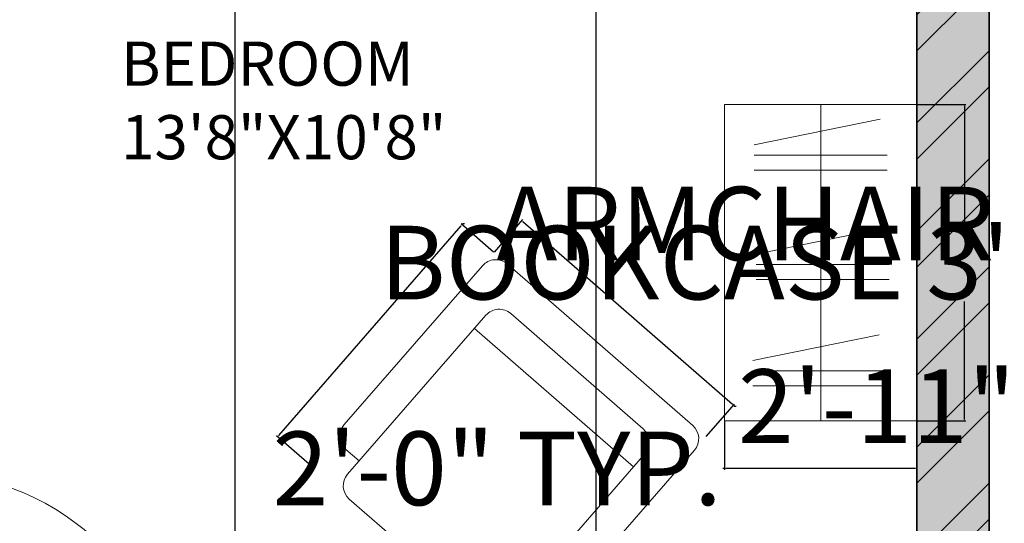
# Model space of a CAD drawing. Units: inches. Extents: x 1086 to 1540, y 3343 to 3848.
# Tile 6 of 8: x 1350 to 1473, y 3661 to 3724. Entities that reach past the tile are written whole.
import ezdxf

# ---------------------------------------------------------------- set-up
doc = ezdxf.new("R2010")
doc.units = ezdxf.units.IN
for name, color, linetype, lineweight in [('00 FURNITURE', 15, 'Continuous', 15), ('A-ANNO-DIMS', 2, 'Continuous', 13), ('A-AREA-IDEN', 7, 'Continuous', 18), ('A-DOOR', 4, 'Continuous', 20), ('A-FLOR-CASE', 8, 'Continuous', 18), ('A-WALL-PATT', 252, 'Continuous', 9), ('WALL', 7, 'Continuous', 35)]:
    doc.layers.add(name, color=color, linetype=linetype, lineweight=lineweight)
doc.styles.get("Standard").update_dxf_attribs({"font": 'arial.ttf'})
doc.dimstyles.get("Standard").update_dxf_attribs({"dimtxt": 9.18, "dimasz": 0.18, "dimexe": 0.18, "dimexo": 0.0625, "dimgap": 0.09, "dimtad": 0, "dimtih": 1, "dimtoh": 1, "dimdec": 1, "dimzin": 0, "dimdsep": 46, "dimlunit": 3, "dimtxsty": 'Standard', "dimcen": 0.09, "dimadec": 0, "dimazin": 0, "dimtfac": 1, "dimtdec": 1, "dimtofl": 0, "dimtmove": 0, "dimatfit": 3, "dimfxl": 1, "dimtolj": 1, "dimtzin": 0, "dimarcsym": 0})

# ---------------------------------------------------------------- blocks, each defined once
blk = doc.blocks.new('DDD')
at = {"layer": '00 FURNITURE'}
for p, q in [((-12579.77, -15859.53), (-12579.77, -15829.05)), ((-12578.77, -15859.53), (-12578.77, -15829.03)), ((-12612.02, -15857.03), (-12612.02, -15862.03)), ((-12611.02, -15857.03), (-12612.02, -15857.03)), ((-12610.52, -15858.03), (-12610.52, -15857.53)), ((-12577.52, -15858.03), (-12577.52, -15857.53)), ((-12577.02, -15857.03), (-12576.02, -15857.03)), ((-12576.02, -15857.03), (-12576.02, -15862.03)), ((-12578.77, -15859.53), (-12579.77, -15859.53)), ((-12610.52, -15861.53), (-12610.52, -15861.03)), ((-12577.52, -15861.53), (-12577.52, -15861.03)), ((-12612.02, -15862.03), (-12611.02, -15862.03)), ((-12576.02, -15862.03), (-12577.02, -15862.03))]:
    blk.add_line(p, q, dxfattribs=at)
for points in [[(-12610.52, -15861.03), (-12610.02, -15861.03, 0.414214), (-12609.52, -15860.53), (-12609.52, -15858.53, 0.414214), (-12610.02, -15858.03), (-12610.52, -15858.03)], [(-12577.52, -15861.03), (-12578.02, -15861.03, -0.414214), (-12578.52, -15860.53), (-12578.52, -15858.53, -0.414214), (-12578.02, -15858.03), (-12577.52, -15858.03)]]:
    blk.add_lwpolyline(points, format="xyb", dxfattribs=at)
for centre, radius, start, end in [((-12578.77, -15859.53), 30.5, 90, 180), ((-12611.02, -15857.53), 0.5, 0, 90), ((-12577.02, -15857.53), 0.5, 90, 180), ((-12611.02, -15861.53), 0.5, 270, 0), ((-12577.02, -15861.53), 0.5, 180, 270)]:
    blk.add_arc(centre, radius, start, end, dxfattribs=at)
blk = doc.blocks.new('chair')
at = {"layer": '00 FURNITURE'}
for p, q in [((1375.85, 3529.75), (1402.12, 3529.75)), ((1373.66, 3525.37), (1373.66, 3527.56)), ((1404.31, 3527.56), (1404.31, 3496.9)), ((1371.47, 3525.37), (1397.74, 3525.37)), ((1395.55, 3525.37), (1395.55, 3499.09)), ((1369.28, 3501.28), (1369.28, 3523.18)), ((1399.93, 3523.18), (1399.93, 3501.28)), ((1397.74, 3499.09), (1371.47, 3499.09)), ((1373.66, 3496.9), (1373.66, 3499.09)), ((1402.12, 3494.71), (1375.85, 3494.71))]:
    blk.add_line(p, q, dxfattribs=at)
for centre, start, end in [((1375.85, 3527.56), 90, 180), ((1402.12, 3527.56), 0, 90), ((1371.47, 3523.18), 90, 180), ((1397.74, 3523.18), 0, 90), ((1371.47, 3501.28), 180, 270), ((1397.74, 3501.28), 270, 0), ((1375.85, 3496.9), 180, 270), ((1402.12, 3496.9), 270, 0)]:
    blk.add_arc(centre, 2.19, start, end, dxfattribs=at)
blk = doc.blocks.new('*D13')
at = {"layer": 'A-ANNO-DIMS', "color": 0, "lineweight": -2, "transparency": 16777216}
for p, q in [((1470.8, 3811.57), (1506.93, 3811.57)), ((1506.75, 3811.39), (1506.75, 3600.35)), ((1506.75, 3379.75), (1506.75, 3590.79)), ((1470.8, 3379.57), (1506.93, 3379.57))]:
    blk.add_line(p, q, dxfattribs=at)
at = {"layer": 'A-ANNO-DIMS', "color": 0, "transparency": 16777216}
for points in [[(1506.72, 3811.39), (1506.78, 3811.39), (1506.75, 3811.57)], [(1506.72, 3379.75), (1506.78, 3379.75), (1506.75, 3379.57)]]:
    blk.add_solid(points, dxfattribs=at)
at = {"layer": 'Defpoints', "color": 0, "transparency": 16777216}
for p in [(1470.74, 3811.57), (1470.74, 3379.57), (1506.75, 3379.57)]:
    blk.add_point(p, dxfattribs=at)
at = {"layer": 'A-ANNO-DIMS', "color": 0, "transparency": 16777216, "insert": (1506.75, 3595.57), "char_height": 9.18, "attachment_point": 5}
blk.add_mtext("\\A1;36'", dxfattribs=at)
blk = doc.blocks.new('BOOKCASE-FRAME')
for p, q in [((24, 39.45), (0, 39.45)), ((12, 39.45), (12, 0)), ((24, 0), (24, 39.45)), ((0, 0), (24, 0))]:
    blk.add_line(p, q)
blk = doc.blocks.new('BOOKCASE-CONTENTS')
for p, q in [((0.85, 6.37), (16.59, 3.17)), ((0, 1.86), (16.59, 1.86)), ((0, 0), (16.59, 0)), ((0.59, -7.26), (16.34, -10.46)), ((-0.25, -11.76), (16.34, -11.76)), ((-0.25, -13.62), (16.34, -13.62)), ((0.99, -20.52), (16.73, -23.72)), ((0.14, -25.02), (16.73, -25.02)), ((0.14, -26.89), (16.73, -26.89))]:
    blk.add_line(p, q)
blk = doc.blocks.new('*D26')
at = {"layer": 'A-ANNO-DIMS', "color": 0, "lineweight": -2, "transparency": 16777216}
for p, q in [((1335.68, 3667.57), (1330.16, 3667.57)), ((1330.34, 3667.39), (1330.34, 3655.85)), ((1330.34, 3634.75), (1330.34, 3646.29)), ((1335.68, 3634.57), (1330.16, 3634.57))]:
    blk.add_line(p, q, dxfattribs=at)
at = {"layer": 'A-ANNO-DIMS', "color": 0, "transparency": 16777216}
for points in [[(1330.31, 3667.39), (1330.37, 3667.39), (1330.34, 3667.57)], [(1330.31, 3634.75), (1330.37, 3634.75), (1330.34, 3634.57)]]:
    blk.add_solid(points, dxfattribs=at)
at = {"layer": 'Defpoints', "color": 0, "transparency": 16777216}
for p in [(1330.34, 3667.57), (1335.74, 3667.57), (1335.74, 3634.57)]:
    blk.add_point(p, dxfattribs=at)
at = {"layer": 'A-ANNO-DIMS', "color": 0, "transparency": 16777216, "insert": (1330.34, 3651.07), "char_height": 9.18, "attachment_point": 5}
blk.add_mtext('\\A1;2\'-9" TYP.', dxfattribs=at)
blk = doc.blocks.new('*D27')
at = {"layer": 'A-ANNO-DIMS', "color": 0, "lineweight": -2, "transparency": 16777216}
for p, q in [((1382.16, 3672.32), (1404.93, 3698.48)), ((1408.96, 3695.2), (1404.91, 3698.73)), ((1405.05, 3698.61), (1405.16, 3698.75)), ((1405.16, 3698.75), (1405.34, 3698.75)), ((1385.96, 3668.77), (1381.9, 3672.3))]:
    blk.add_line(p, q, dxfattribs=at)
at = {"layer": 'A-ANNO-DIMS', "color": 0, "transparency": 16777216}
for points in [[(1404.9, 3698.5), (1404.95, 3698.46), (1405.05, 3698.61)], [(1382.14, 3672.34), (1382.18, 3672.3), (1382.04, 3672.18)]]:
    blk.add_solid(points, dxfattribs=at)
at = {"layer": 'Defpoints', "color": 0, "transparency": 16777216}
for p in [(1405.05, 3698.61), (1409.01, 3695.16), (1386, 3668.73)]:
    blk.add_point(p, dxfattribs=at)
at = {"layer": 'A-ANNO-DIMS', "color": 0, "transparency": 16777216, "insert": (1473.23, 3698.75), "char_height": 9.18, "attachment_point": 5}
blk.add_mtext('\\A1;ARMCHAIR 2\'-11" TYP.', dxfattribs=at)
blk = doc.blocks.new('*D28')
at = {"layer": 'A-ANNO-DIMS', "color": 0, "lineweight": -2, "transparency": 16777216}
for p, q in [((1409.05, 3695.21), (1412.58, 3699.26)), ((1412.6, 3699.01), (1438.75, 3676.24)), ((1435.48, 3672.2), (1439.01, 3676.26)), ((1438.89, 3676.12), (1439.02, 3676)), ((1439.02, 3676), (1439.2, 3676))]:
    blk.add_line(p, q, dxfattribs=at)
at = {"layer": 'A-ANNO-DIMS', "color": 0, "transparency": 16777216}
for points in [[(1412.62, 3699.03), (1412.58, 3698.98), (1412.46, 3699.13)], [(1438.77, 3676.26), (1438.73, 3676.22), (1438.89, 3676.12)]]:
    blk.add_solid(points, dxfattribs=at)
at = {"layer": 'Defpoints', "color": 0, "transparency": 16777216}
for p in [(1409.01, 3695.16), (1438.89, 3676.12), (1435.44, 3672.16)]:
    blk.add_point(p, dxfattribs=at)
at = {"layer": 'A-ANNO-DIMS', "color": 0, "transparency": 16777216, "insert": (1470.92, 3676), "char_height": 9.18, "attachment_point": 5}
blk.add_mtext('\\A1;2\'-11" TYP.', dxfattribs=at)
blk = doc.blocks.new('*D31')
at = {"layer": 'A-ANNO-DIMS', "color": 0, "lineweight": -2, "transparency": 16777216}
for p, q in [((1461.8, 3713.61), (1467.84, 3713.61)), ((1467.66, 3713.43), (1467.66, 3698.73)), ((1467.66, 3674.34), (1467.66, 3689.04)), ((1461.8, 3674.16), (1467.84, 3674.16))]:
    blk.add_line(p, q, dxfattribs=at)
at = {"layer": 'A-ANNO-DIMS', "color": 0, "transparency": 16777216}
for points in [[(1467.63, 3713.43), (1467.69, 3713.43), (1467.66, 3713.61)], [(1467.63, 3674.34), (1467.69, 3674.34), (1467.66, 3674.16)]]:
    blk.add_solid(points, dxfattribs=at)
at = {"layer": 'Defpoints', "color": 0, "transparency": 16777216}
for p in [(1461.74, 3713.61), (1461.74, 3674.16), (1467.66, 3674.16)]:
    blk.add_point(p, dxfattribs=at)
at = {"layer": 'A-ANNO-DIMS', "color": 0, "transparency": 16777216, "insert": (1467.66, 3693.89), "char_height": 9.18, "attachment_point": 5}
blk.add_mtext('\\A1;BOOKCASE 3\'-3 1/2" TYP.', dxfattribs=at)
blk = doc.blocks.new('*D32')
at = {"layer": 'A-ANNO-DIMS', "color": 0, "lineweight": -2, "transparency": 16777216}
for p, q in [((1437.74, 3674.1), (1437.74, 3668.06)), ((1461.74, 3674.1), (1461.74, 3668.06)), ((1437.74, 3668.24), (1437.56, 3668.24)), ((1461.56, 3668.24), (1437.92, 3668.24))]:
    blk.add_line(p, q, dxfattribs=at)
at = {"layer": 'A-ANNO-DIMS', "color": 0, "transparency": 16777216}
for points in [[(1437.92, 3668.27), (1437.92, 3668.21), (1437.74, 3668.24)], [(1461.56, 3668.27), (1461.56, 3668.21), (1461.74, 3668.24)]]:
    blk.add_solid(points, dxfattribs=at)
at = {"layer": 'Defpoints', "color": 0, "transparency": 16777216}
for p in [(1437.74, 3674.16), (1461.74, 3674.16), (1437.74, 3668.24)]:
    blk.add_point(p, dxfattribs=at)
at = {"layer": 'A-ANNO-DIMS', "color": 0, "transparency": 16777216, "insert": (1409.41, 3668.24), "char_height": 9.18, "attachment_point": 5}
blk.add_mtext('\\A1;2\'-0" TYP.', dxfattribs=at)
blk = doc.blocks.new('*D70')
at = {"layer": 'A-ANNO-DIMS', "color": 0, "lineweight": -2, "transparency": 16777216}
for p, q in [((1376.74, 3634.63), (1376.74, 3834.75)), ((1376.92, 3834.57), (1386.95, 3834.57)), ((1421.56, 3834.57), (1411.53, 3834.57)), ((1421.74, 3634.63), (1421.74, 3834.75))]:
    blk.add_line(p, q, dxfattribs=at)
at = {"layer": 'A-ANNO-DIMS', "color": 0, "transparency": 16777216}
for points in [[(1376.92, 3834.6), (1376.92, 3834.54), (1376.74, 3834.57)], [(1421.56, 3834.6), (1421.56, 3834.54), (1421.74, 3834.57)]]:
    blk.add_solid(points, dxfattribs=at)
at = {"layer": 'Defpoints', "color": 0, "transparency": 16777216}
for p in [(1421.74, 3834.57), (1376.74, 3634.57), (1421.74, 3634.57)]:
    blk.add_point(p, dxfattribs=at)
at = {"layer": 'A-ANNO-DIMS', "color": 0, "transparency": 16777216, "insert": (1399.24, 3834.57), "char_height": 9.18, "attachment_point": 5}
blk.add_mtext('\\A1;3\'-9"', dxfattribs=at)

msp = doc.modelspace()

# ---------------------------------------------------------------- hatches: boundary and pattern name
at = {"layer": 'A-WALL-PATT'}
h = msp.add_hatch(dxfattribs=at)
h.set_pattern_fill('ANSI32', color=256)
h.paths.add_polyline_path([(1234.55, 3811.57), (1234.55, 3811.57), (1194.74, 3811.57), (1194.74, 3622.57), (1203.74, 3622.57), (1203.74, 3634.57), (1218.33, 3634.57), (1218.33, 3638.57), (1203.74, 3638.57), (1203.74, 3802.57), (1234.55, 3802.57)])
h.paths.add_polyline_path([(1371.06, 3811.57), (1371.06, 3811.57), (1282.55, 3811.57), (1282.55, 3802.57), (1331.74, 3802.57), (1331.74, 3634.57), (1335.74, 3634.57), (1335.74, 3639.57), (1335.74, 3802.57), (1371.06, 3802.57)])
h.paths.add_polyline_path([(1470.74, 3811.57), (1419.06, 3811.57), (1419.06, 3802.57), (1461.74, 3802.57), (1461.74, 3638.57), (1461.74, 3548.57), (1425.74, 3548.57), (1425.74, 3582.21), (1421.74, 3582.21), (1421.74, 3548.57), (1376.74, 3548.57), (1376.74, 3602.57), (1373.71, 3602.57), (1372.74, 3602.57), (1372.74, 3544.57), (1461.74, 3544.57), (1461.74, 3379.57), (1470.74, 3379.57)])
h.paths.add_polyline_path([(1203.74, 3582.57), (1295.74, 3582.57), (1295.74, 3586.57), (1203.74, 3586.57), (1203.74, 3598.57), (1194.74, 3598.57), (1194.74, 3379.57), (1326.74, 3379.57), (1326.74, 3388.57), (1322.74, 3388.57), (1203.74, 3388.57), (1203.74, 3451.57), (1234.74, 3451.57), (1234.74, 3455.57), (1203.74, 3455.57), (1203.74, 3479.57), (1203.74, 3544.57), (1227.74, 3544.57), (1253.74, 3544.57), (1253.74, 3548.57), (1203.74, 3548.57)])
h.paths.add_polyline_path([(1461.74, 3638.57), (1371.74, 3638.57), (1371.74, 3634.57), (1372.74, 3634.57), (1372.74, 3632.57), (1376.74, 3632.57), (1376.74, 3634.57), (1421.74, 3634.57), (1421.74, 3606.21), (1425.74, 3606.21), (1425.74, 3634.57), (1461.74, 3634.57)])
h.paths.add_polyline_path([(1295.74, 3638.57), (1266.33, 3638.57), (1266.33, 3634.57), (1292.74, 3634.57), (1295.74, 3634.57)])
h.paths.add_polyline_path([(1322.74, 3548.57), (1318.74, 3548.57), (1318.74, 3455.57), (1282.74, 3455.57), (1282.74, 3451.57), (1318.74, 3451.57), (1318.74, 3420.07), (1322.74, 3420.07)], flags=17)
at = {"layer": 'A-WALL-PATT', "transparency": 33554559}
h = msp.add_hatch(color=256, dxfattribs=at)
h.dxf.hatch_style = 1
h.paths.add_polyline_path([(1234.55, 3811.57), (1234.55, 3811.57), (1194.74, 3811.57), (1194.74, 3622.57), (1203.74, 3622.57), (1203.74, 3634.57), (1218.33, 3634.57), (1218.33, 3638.57), (1203.74, 3638.57), (1203.74, 3802.57), (1234.55, 3802.57)])
h.paths.add_polyline_path([(1371.06, 3811.57), (1371.06, 3811.57), (1282.55, 3811.57), (1282.55, 3802.57), (1331.74, 3802.57), (1331.74, 3634.57), (1335.74, 3634.57), (1335.74, 3639.57), (1335.74, 3802.57), (1371.06, 3802.57)])
h.paths.add_polyline_path([(1470.74, 3811.57), (1419.06, 3811.57), (1419.06, 3802.57), (1461.74, 3802.57), (1461.74, 3638.57), (1461.74, 3548.57), (1425.74, 3548.57), (1425.74, 3582.21), (1421.74, 3582.21), (1421.74, 3548.57), (1376.74, 3548.57), (1376.74, 3602.57), (1372.74, 3602.57), (1372.74, 3544.57), (1461.74, 3544.57), (1461.74, 3379.57), (1470.74, 3379.57)])
h.paths.add_polyline_path([(1203.74, 3544.57), (1227.74, 3544.57), (1253.74, 3544.57), (1253.74, 3548.57), (1203.74, 3548.57), (1203.74, 3582.57), (1295.74, 3582.57), (1295.74, 3586.57), (1203.74, 3586.57), (1203.74, 3598.57), (1194.74, 3598.57), (1194.74, 3379.57), (1326.74, 3379.57), (1326.74, 3388.57), (1322.74, 3388.57), (1203.74, 3388.57), (1203.74, 3451.57), (1234.74, 3451.57), (1234.74, 3455.57), (1203.74, 3455.57)])
h.paths.add_polyline_path([(1413.74, 3388.57), (1413.74, 3388.57), (1374.74, 3388.57), (1374.74, 3383.18), (1374.74, 3383.18), (1374.74, 3379.57), (1413.74, 3379.57)], flags=17)
h.paths.add_polyline_path([(1322.74, 3548.57), (1318.74, 3548.57), (1318.74, 3455.57), (1282.74, 3455.57), (1282.74, 3451.57), (1318.74, 3451.57), (1318.74, 3420.07), (1322.74, 3420.07)], flags=17)
h.paths.add_polyline_path([(1295.74, 3638.57), (1266.33, 3638.57), (1266.33, 3634.57), (1292.74, 3634.57), (1295.74, 3634.57)])
h.paths.add_polyline_path([(1461.74, 3638.57), (1371.74, 3638.57), (1371.74, 3634.57), (1372.74, 3634.57), (1372.74, 3632.57), (1376.74, 3632.57), (1376.74, 3634.57), (1421.74, 3634.57), (1421.74, 3606.21), (1425.74, 3606.21), (1425.74, 3634.57), (1461.74, 3634.57)])

# ---------------------------------------------------------------- linework, layer by layer
at = {"layer": 'WALL'}
for p, q in [((1470.74, 3811.57), (1470.74, 3379.57)), ((1461.74, 3802.57), (1461.74, 3638.57))]:
    msp.add_line(p, q, dxfattribs=at)

# ---------------------------------------------------------------- block references
at = {"layer": '00 FURNITURE', "xscale": -1, "rotation": 228.9612801357977}
msp.add_blockref('chair', (-2148.96, 4930.45), dxfattribs=at)
at = {"layer": 'A-DOOR', "xscale": -1}
msp.add_blockref('DDD', (-11240.28, 19496.6), dxfattribs=at)
at = {"layer": 'A-FLOR-CASE', "rotation": 180}
msp.add_blockref('BOOKCASE-FRAME', (1461.74, 3713.61), dxfattribs=at)
at = {"layer": 'A-FLOR-CASE', "extrusion": (0, 0, -1), "zscale": -1}
msp.add_blockref('BOOKCASE-CONTENTS', (-1458.02, 3705.42), dxfattribs=at)

# ---------------------------------------------------------------- texts
at = {"layer": 'A-AREA-IDEN', "insert": (1362.5, 3721.44), "char_height": 8, "attachment_point": 1}
msp.add_mtext_dynamic_manual_height_columns('{\\H0.6875x;BEDROOM\\P13\'8"X10\'8"\\H1.1818x; }  ', width=58.9878, gutter_width=0, heights=[37.04], dxfattribs=at)

# ---------------------------------------------------------------- dimensions: what is measured, and where the dimension line sits
at = {"layer": 'A-ANNO-DIMS'}
dim = msp.add_linear_dim(base=(1421.74, 3834.57), p1=(1376.74, 3634.57), p2=(1421.74, 3634.57), dimstyle='Standard', override={"dimdec": 1, "dimlfac": 1, "dimrnd": 0, "dimzin": 1, "dimdsep": 46, "dimlunit": 4, "dimfrac": 2}, dxfattribs=at)
dim.commit()
dim.dimension.update_dxf_attribs({"geometry": '*D70', "text_midpoint": (1399.24, 3834.57)})
dim = msp.add_linear_dim(base=(1506.75, 3379.57), p1=(1470.74, 3811.57), p2=(1470.74, 3379.57), angle=90, dimstyle='Standard', override={"dimclrd": 0, "dimclre": 0, "dimclrt": 0}, dxfattribs=at)
dim.commit()
dim.dimension.update_dxf_attribs({"geometry": '*D13', "text_midpoint": (1506.75, 3595.57)})
for base, p1, p2, angle, text, picture, middle in [((1467.6583, 3674.1617), (1461.7404, 3713.6137), (1461.7404, 3674.1617), 270, 'BOOKCASE <> TYP.', '*D31', (1467.6583, 3693.8877)), ((1405.05, 3698.61), (1386, 3668.73), (1409.01, 3695.16), 48.9613, 'ARMCHAIR <> TYP.', '*D27', (1473.23, 3698.75)), ((1438.89, 3676.12), (1409.01, 3695.16), (1435.44, 3672.16), 318.9613, '<> TYP.', '*D28', (1470.92, 3676)), ((1437.74, 3668.24), (1461.74, 3674.16), (1437.74, 3674.16), 180, '<> TYP.', '*D32', (1409.41, 3668.24)), ((1330.34, 3667.57), (1335.74, 3634.57), (1335.74, 3667.57), 90, '<> TYP.', '*D26', (1330.34, 3651.07))]:
    dim = msp.add_linear_dim(base=base, p1=p1, p2=p2, angle=angle, text=text, dimstyle='Standard', override={"dimdec": 1, "dimlfac": 1, "dimrnd": 0, "dimzin": 1, "dimdsep": 46, "dimlunit": 4, "dimfrac": 2}, dxfattribs=at)
    dim.commit()
    dim.dimension.update_dxf_attribs({"geometry": picture, "text_midpoint": middle})

doc.saveas('drawing.dxf')
